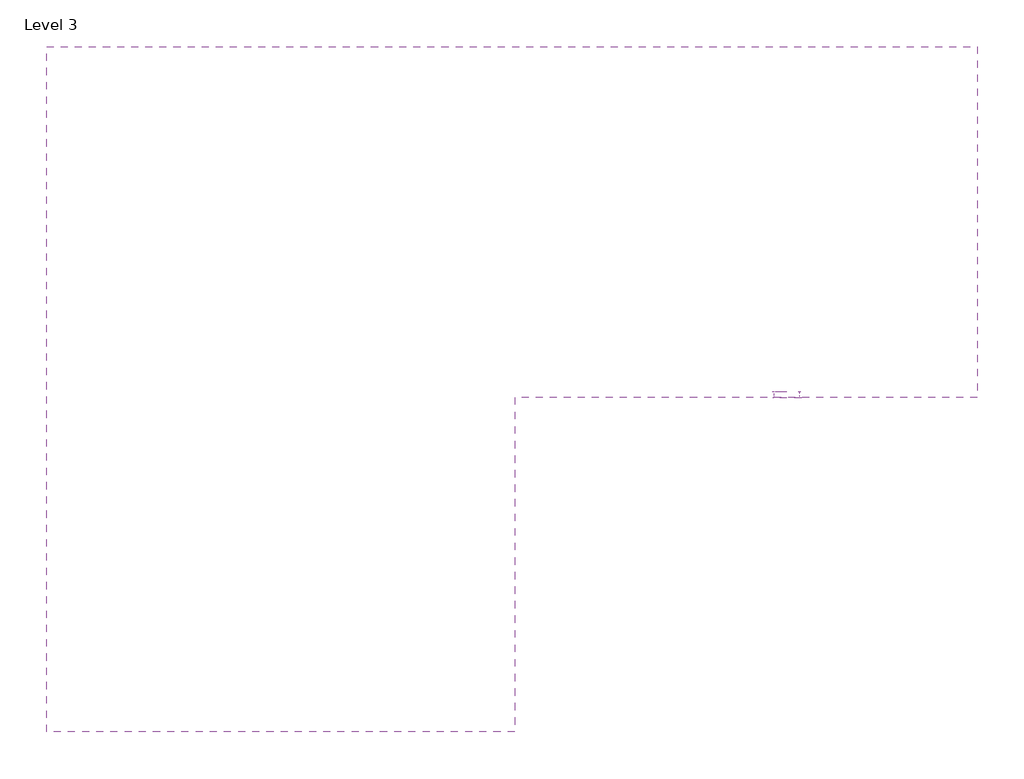
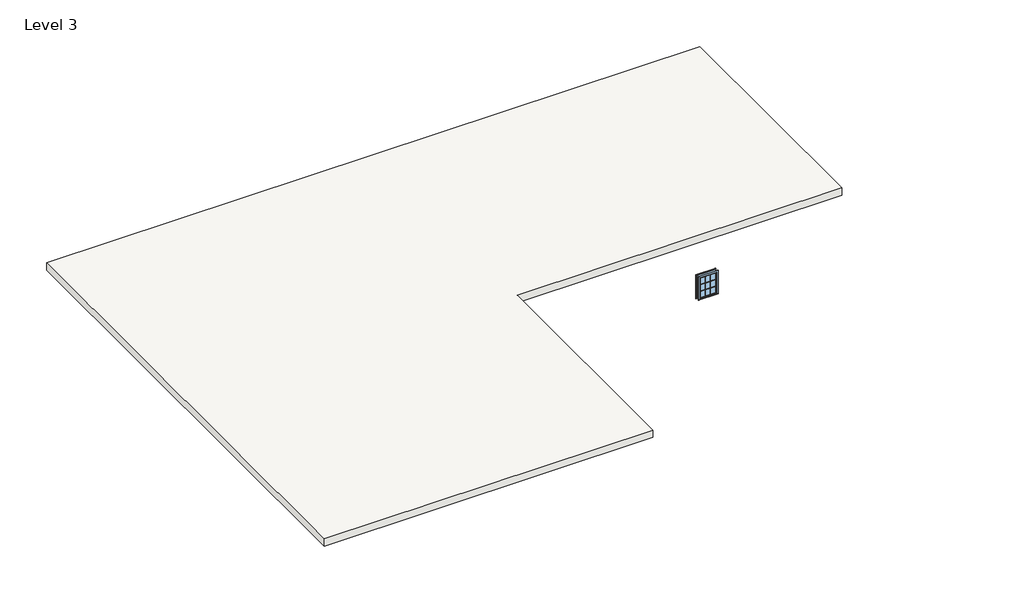
# One storey, incomplete: 1 slab, 1 window.
"""IFC4 building model written with IfcOpenShell, lengths in millimetres."""

from ifc_helpers import new_model, si_unit, frame, origin, place, context, project, spatial, polyline, outline, extrude, transform, mapped, element, save
from components import window_ddc5d35f

model = new_model("IFC4")

# Units and contexts
model_context = context("Model", 3, world=origin())
ifc_project = project(units=[si_unit("LENGTHUNIT", "METRE", prefix="MILLI")], contexts=[model_context])

# Site, building, storey
site = spatial("IfcSite", under=ifc_project)
building = spatial("IfcBuilding", under=site)
storey = spatial("IfcBuildingStorey", under=building, Name="Level 3", Elevation=7048.0)

# Slab
placement = place(None, origin())
element("IfcSlab", 1, ObjectType="Generic Floor - 400mm", at=placement, inside=storey, context=model_context, shape_type="SweptSolid", body=[
    extrude(outline(polyline([(15697.920453, 15683.5992031), (15697.920453, 2788.3992031), (-1302.079547, 2788.3992031), (-1302.079547, -9516.4007969), (-18502.079547, -9516.4007969), (-18502.079547, 15683.5992031), (15697.920453, 15683.5992031)])), frame((0.0, 0.0, 11696.0), z_axis=(0.0, 0.0, 1.0), x_axis=(1.0, 0.0, 0.0)), (0.0, 0.0, 1.0), 400.0),
])

# Window
window_shape = window_ddc5d35f(model_context)
element("IfcWindow", 2, ObjectType="Casement 3x3 with Trim : 36\" x 48\"", at=placement, inside=storey, context=model_context, shape_type="MappedRepresentation", body=[
    mapped(window_shape, transform((8697.920453, 2888.3992031, 7600.0), x_axis=(-1.0, 0.0, 0.0), y_axis=(0.0, -1.0, 0.0), z_axis=(0.0, 0.0, 1.0))),
])

save(model, "model.ifc")

# Revit data of these elements
# Type "Generic Floor - 400mm"
#   Function = 0
#   Layers, outside or top first: 1' - 3.74803" no material (function 1)
# Type "Casement 3x3 with Trim : 36\" x 48\""
#   Type Mark = "19"
#   Construction Type Id = "GSP4R"
#   Assembly Code = "B2020100"
#   Analytic Construction = "1/8 in Pilkington single glazing"
#   Visual Light Transmittance = 0.9
#   Solar Heat Gain Coefficient = 0.78
#   Heat Transfer Coefficient (U) = 3.6886 W/(m²·K)
#   Height = 4' - 0"
#   Default Sill Height = 3' - 0"
#   Trim Projection - Ext. = 0' - 0 1/2"
#   Trim Projection - Int. = 0' - 0 3/4"
#   Trim Width - Exterior = 0' - 3 1/2"
#   Trim Width - Interior = 0' - 3 1/2"
#   Width = 3' - 0"
#   Window Inset = 0' - 0 3/4"
#   Define Thermal Properties by = 1
#   Glass Pane Material = Glass
#   Sash Material = Sash
#   Trim Exterior Material = Trim
#   Trim Interior Material = Trim
#   Wall Closure = (empty or 0)
# Element 1 (IfcSlab, "Generic Floor - 400mm")
#   Height Offset From Level = 16' - 6.74016"
#   Phase Created = New Construction
#   Materials on its faces: "Default Roof"
# Element 2 (IfcWindow, "Casement 3x3 with Trim : 36\" x 48\"")
#   Mark = "7"
#   Phase Created = New Construction
#   Materials on its faces: "Sash", "Glass", "Trim"
# Materials
#   "Glass": class "Glass", colour RGB 218 227 224, transparency 0.85, Description = "Soda Lime Glass", Cost = 0
#   "Sash": class "Wood", colour RGB 136 99 55, transparency 0
#   "Trim": class "Wood", colour RGB 224 178 126, transparency 0
#   "Default Roof": colour RGB 80 80 80, transparency 0
